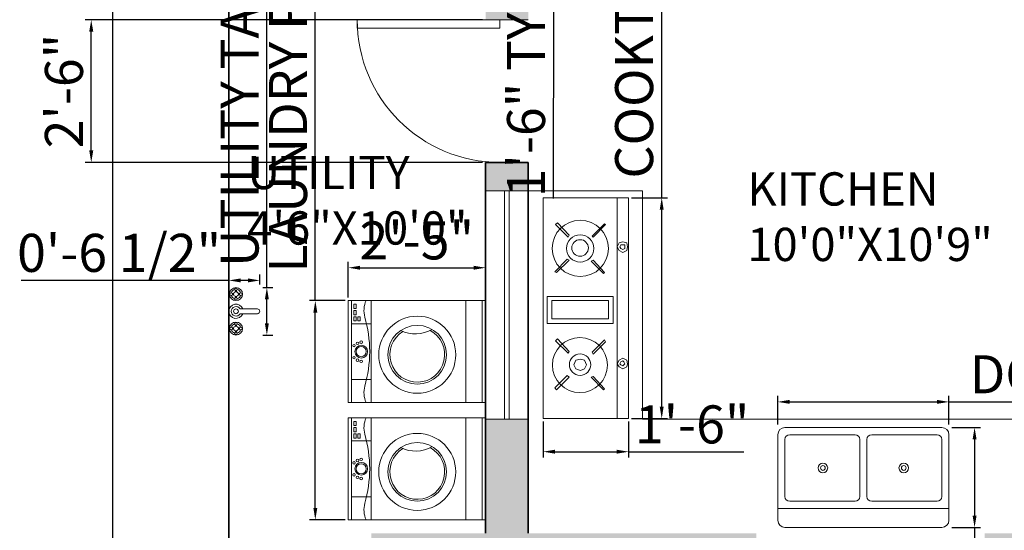
# Model space of a CAD drawing. Units: inches. Extents: x 4732 to 5926, y 2665 to 3255.
# Tile 2 of 8: x 4774 to 4982, y 2827 to 2934. Entities that reach past the tile are written whole.
import ezdxf

# ---------------------------------------------------------------- set-up
doc = ezdxf.new("R2010")
doc.units = ezdxf.units.IN
for name, color, linetype, lineweight in [('A-ANNO-DIMS', 2, 'Continuous', 18), ('A-AREA-IDEN', 7, 'Continuous', 18), ('A-DOOR', 3, 'Continuous', 18), ('A-EQPM', 8, 'Continuous', 18), ('A-FLOR-CASE', 7, 'Continuous', 18), ('A-GLAZ', 4, 'Continuous', 18), ('A-WALL', 7, 'Continuous', 35), ('A-WALL-PATT', 8, 'Continuous', 13), ('C-PROP', 7, 'Continuous', 35), ('Сантехника', 7, 'Continuous', 18)]:
    doc.layers.add(name, color=color, linetype=linetype, lineweight=lineweight)
doc.styles.get("Standard").update_dxf_attribs({"font": 'arial.ttf'})
doc.dimstyles.new('ISO-25', dxfattribs={"dimtxt": 8, "dimasz": 2.5, "dimexe": 1.25, "dimexo": 0.625, "dimtad": 1, "dimdec": 1, "dimlunit": 3, "dimtxsty": 'Standard', "dimcen": 2.5, "dimadec": 0, "dimazin": 0, "dimtfac": 1, "dimtdec": 1, "dimtmove": 0, "dimatfit": 3, "dimfxl": 1, "dimarcsym": 0})

# ---------------------------------------------------------------- blocks, each defined once
blk = doc.blocks.new('Sink-double - 36 in top')
for p, q in [((-18, -4), (18, -4)), ((-0.75, -18.5), (-0.75, -6.5)), ((0.75, -6.5), (0.75, -18.5))]:
    blk.add_line(p, q)
for points in [[(-16.5, 0), (16.5, 0)], [(-18, -19.5), (-18, -1.5)], [(18, -1.5), (18, -19.5)], [(-15.5, -5.5), (-1.75, -5.5)], [(1.75, -5.5), (15.5, -5.5)], [(-16.5, -18.5), (-16.5, -6.5)], [(16.5, -6.5), (16.5, -18.5)], [(-1.75, -19.5), (-15.5, -19.5)], [(15.5, -19.5), (1.75, -19.5)], [(16.5, -21), (-16.5, -21)]]:
    blk.add_lwpolyline(points)
for centre, radius in [((-8.5, -12.5), 1), ((-8.5, -12.5), 0.5), ((8.5, -12.5), 1), ((8.5, -12.5), 0.5)]:
    blk.add_circle(centre, radius)
for centre, radius, start, end in [((-16.5, -1.5), 1.5, 90, 180), ((16.5, -1.5), 1.5, 0, 90), ((-15.5, -6.5), 1, 90, 180), ((-1.75, -6.5), 1, 0, 90), ((1.75, -6.5), 1, 90, 180), ((15.5, -6.5), 1, 0, 90), ((-15.5, -18.5), 1, 180, 270), ((-1.75, -18.5), 1, 270, 0), ((1.75, -18.5), 1, 180, 270), ((15.5, -18.5), 1, 270, 0), ((-16.5, -19.5), 1.5, 180, 270), ((16.5, -19.5), 1.5, 270, 0)]:
    blk.add_arc(centre, radius, start, end)
blk = doc.blocks.new('wash')
at = {"layer": 'Сантехника'}
for p, q in [((4817.13, 2840.92), (4788.24, 2840.92)), ((4788.24, 2819.46), (4788.24, 2840.92)), ((4788.93, 2819.46), (4788.93, 2840.92)), ((4793.08, 2819.46), (4793.08, 2840.92)), ((4812.98, 2819.46), (4812.98, 2840.92)), ((4816.44, 2819.46), (4816.44, 2840.92)), ((4817.13, 2819.46), (4817.13, 2840.92)), ((4793.08, 2836.07), (4788.93, 2836.07)), ((4793.08, 2824.31), (4788.93, 2824.31)), ((4817.13, 2819.46), (4788.24, 2819.46)), ((4817.13, 2816.27), (4788.24, 2816.27)), ((4788.24, 2794.82), (4788.24, 2816.27)), ((4788.93, 2794.82), (4788.93, 2816.27)), ((4793.08, 2794.82), (4793.08, 2816.27)), ((4812.98, 2794.82), (4812.98, 2816.27)), ((4816.44, 2794.82), (4816.44, 2816.27)), ((4817.13, 2794.82), (4817.13, 2816.27)), ((4793.08, 2811.43), (4788.93, 2811.43)), ((4793.08, 2799.66), (4788.93, 2799.66)), ((4817.13, 2794.82), (4788.24, 2794.82))]:
    blk.add_line(p, q, dxfattribs=at)
for points in [[(4789.4, 2839.27), (4789.4, 2840.17), (4789.9, 2840.17), (4789.9, 2839.27)], [(4789.4, 2837.95), (4789.4, 2838.85), (4789.9, 2838.85), (4789.9, 2837.95)], [(4789.4, 2836.64), (4789.4, 2837.53), (4789.9, 2837.53), (4789.9, 2836.64)], [(4790.27, 2836.64), (4790.27, 2837.53), (4790.77, 2837.53), (4790.77, 2836.64)], [(4789.4, 2814.62), (4789.4, 2815.52), (4789.9, 2815.52), (4789.9, 2814.62)], [(4789.4, 2813.31), (4789.4, 2814.2), (4789.9, 2814.2), (4789.9, 2813.31)], [(4789.4, 2811.99), (4789.4, 2812.89), (4789.9, 2812.89), (4789.9, 2811.99)], [(4790.27, 2811.99), (4790.27, 2812.89), (4790.77, 2812.89), (4790.77, 2811.99)]]:
    blk.add_lwpolyline(points, close=True, dxfattribs=at)
for centre, radius in [((4802.77, 2829.54), 8.1), ((4802.77, 2829.54), 6.17), ((4790.19, 2831.93), 0.271), ((4790.98, 2832.18), 0.271), ((4789.46, 2831.45), 0.271), ((4790.98, 2830.19), 1.34), ((4790.98, 2830.19), 1.07), ((4789.46, 2828.92), 0.271), ((4790.19, 2828.4), 0.271), ((4790.98, 2828.15), 0.271), ((4802.77, 2804.9), 8.1), ((4802.77, 2804.9), 6.17), ((4789.46, 2806.8), 0.271), ((4790.19, 2807.28), 0.271), ((4790.98, 2807.53), 0.271), ((4790.98, 2805.55), 1.34), ((4790.98, 2805.55), 1.07), ((4789.46, 2804.27), 0.271), ((4790.19, 2803.75), 0.271), ((4790.98, 2803.5), 0.271)]:
    blk.add_circle(centre, radius, dxfattribs=at)
for centre, radius, start, end in [((4796.44, 2838.85), 4.89, 154.895, 196.6068), ((4762.87, 2829.66), 29.92, 1.0206, 15.0937), ((4802.77, 2829.54), 5.77, 121.8067, 62.1506), ((4802.39, 2840.74), 6.83, 243.19, 300.7673), ((4762.87, 2830.72), 29.92, 344.9063, 358.9794), ((4796.44, 2821.54), 4.89, 163.3932, 205.105), ((4796.44, 2814.2), 4.89, 154.895, 196.6068), ((4762.87, 2805.01), 29.92, 1.0206, 15.0937), ((4802.77, 2804.9), 5.77, 121.8067, 62.1506), ((4802.39, 2816.1), 6.83, 243.19, 300.7673), ((4762.87, 2806.08), 29.92, 344.9063, 358.9794), ((4796.44, 2796.89), 4.89, 163.3932, 205.105)]:
    blk.add_arc(centre, radius, start, end, dxfattribs=at)
blk = doc.blocks.new('gas 1')
for points in [[(35.93, -1.87), (35.93, 0), (0, 0), (0, -1.87)], [(8.12, -0.94), (8.44, -1.56), (8.91, -1.87), (9.53, -1.56), (9.84, -0.94), (9.53, -0.31), (8.91, -0.16), (8.44, -0.31)], [(8.59, -0.94), (8.75, -1.25), (8.91, -1.41), (9.22, -1.25), (9.37, -0.94), (9.22, -0.78), (8.91, -0.62), (8.75, -0.78)], [(27.03, -0.94), (27.34, -1.56), (27.97, -1.87), (28.59, -1.56), (28.75, -0.94), (28.59, -0.31), (27.97, -0.16), (27.34, -0.31)], [(27.5, -0.94), (27.65, -1.25), (27.97, -1.41), (28.28, -1.25), (28.28, -0.94), (28.28, -0.62), (27.97, -0.62), (27.65, -0.62)], [(19.84, -13.28), (15.47, -13.28), (15.47, -2.5), (19.84, -2.5)], [(4.84, -3.91), (4.69, -4.06), (6.72, -6.09), (6.87, -5.78)], [(12.81, -3.91), (12.5, -3.75), (10.47, -5.78), (10.78, -5.94)], [(19.22, -12.5), (16.25, -12.5), (16.25, -3.28), (19.22, -3.28)], [(23.75, -3.91), (23.59, -4.06), (25.62, -6.09), (25.78, -5.78)], [(31.71, -3.91), (31.56, -3.75), (29.53, -5.78), (29.68, -5.94)], [(7.81, -7.81), (8.12, -8.59), (8.75, -8.91), (9.53, -8.59), (9.69, -7.81), (9.53, -7.19), (8.75, -6.87), (8.12, -7.19)], [(7.03, -10), (6.72, -9.69), (4.69, -11.72), (5, -12.03)], [(12.97, -11.56), (10.94, -9.69), (10.62, -9.84), (12.65, -11.87)], [(23.75, -11.72), (23.9, -12.03), (25.93, -10), (25.78, -9.69)], [(31.87, -11.56), (29.84, -9.69), (29.53, -9.84), (31.56, -11.87)]]:
    blk.add_lwpolyline(points, close=True)
blk.add_lwpolyline([(35.93, -1.87), (35.93, -13.9), (0, -13.9), (0, -1.87)])
for centre, radius in [((8.7, -7.92), 4.48), ((27.7, -7.86), 4.58), ((8.77, -7.89), 1.74), ((27.69, -7.89), 2.22), ((27.76, -7.89), 1.35)]:
    blk.add_circle(centre, radius)
blk = doc.blocks.new('*U19')
for p, q in [((0, 0), (0, -6)), ((30, 0), (30, -6))]:
    blk.add_line(p, q)
blk.add_lwpolyline([(0, 0), (0, 30), (1.75, 30), (1.75, 0)], close=True)
blk.add_arc((0, 0), 30, 0, 90)
blk = doc.blocks.new('*D28')
at = {"layer": 'A-ANNO-DIMS', "color": 0, "lineweight": -2, "transparency": 16777216}
for p, q in [((4817.76, 3215.93), (4792.67, 3215.93)), ((4793.92, 3213.43), (4793.92, 2738.43)), ((4817.76, 2735.93), (4792.67, 2735.93))]:
    blk.add_line(p, q, dxfattribs=at)
at = {"layer": 'A-ANNO-DIMS', "color": 0, "transparency": 16777216}
for points in [[(4793.5, 3213.43), (4794.33, 3213.43), (4793.92, 3215.93)], [(4793.5, 2738.43), (4794.33, 2738.43), (4793.92, 2735.93)]]:
    blk.add_solid(points, dxfattribs=at)
at = {"layer": 'Defpoints', "color": 0, "transparency": 16777216}
for p in [(4818.38, 3215.93), (4793.92, 2735.93), (4818.38, 2735.93)]:
    blk.add_point(p, dxfattribs=at)
at = {"layer": 'A-ANNO-DIMS', "color": 0, "transparency": 16777216, "insert": (4789.21, 2975.93), "char_height": 8, "attachment_point": 5, "rotation": 90}
blk.add_mtext("40'", dxfattribs=at)
blk = doc.blocks.new('Faucet - Bathroom top')
for p, q in [((-4.107, 0.125), (-4.375, 0.125)), ((-3.75, 0.4788), (-3.75, 0.75)), ((-3.5, 0.482), (-3.5, 0.75)), ((-3.1461, 0.125), (-2.875, 0.125)), ((3.143, 0.125), (2.875, 0.125)), ((3.5, 0.4788), (3.5, 0.75)), ((3.75, 0.482), (3.75, 0.75)), ((4.1039, 0.125), (4.375, 0.125)), ((-4.1039, -0.125), (-4.375, -0.125)), ((-3.75, -0.4821), (-3.75, -0.75)), ((-3.5, -0.4789), (-3.5, -0.75)), ((-3.143, -0.125), (-2.875, -0.125)), ((-0.5, -0.8639), (-0.5, -4.5)), ((0.5, -4.5), (0.5, -0.8631)), ((3.1461, -0.125), (2.875, -0.125)), ((3.5, -0.4821), (3.5, -0.75)), ((3.75, -0.4789), (3.75, -0.75)), ((4.107, -0.125), (4.375, -0.125))]:
    blk.add_line(p, q)
for centre, radius in [((-3.625, 0), 1.375), ((-4.625, 0), 0.2795), ((-3.625, 0), 0.5), ((-3.625, 1), 0.2795), ((-2.625, 0), 0.2795), ((0, 0), 0.5), ((3.625, 0), 1.375), ((2.625, 0), 0.2795), ((3.625, 0), 0.5), ((3.625, 1), 0.2795), ((4.625, 0), 0.2795), ((-3.625, -1), 0.2795), ((3.625, -1), 0.2795)]:
    blk.add_circle(centre, radius)
for centre, radius, start, end in [((-3.625, 0), 1, 105.2407, 164.2093), ((-3.625, 0), 1, 16.44125, 74.07887), ((0, 0), 1.5, 289.6514, 250.3603), ((0, 0), 1, 300.3431, 239.7554), ((3.625, 0), 1, 106.12, 164.0884), ((3.625, 0), 1, 16.23422, 73.90469), ((-3.625, 0), 1, 196.2342, 253.9047), ((-3.625, 0), 1, 286.12, 344.0884), ((3.625, 0), 1, 196.4413, 254.0789), ((3.625, 0), 1, 285.2407, 344.2093), ((0, -4.5), 0.5, 180, 0)]:
    blk.add_arc(centre, radius, start, end)
blk = doc.blocks.new('GLAZ-UNIT-48IN')
for p, q in [((0, 1), (48, 1)), ((0, 0), (48, 0))]:
    blk.add_line(p, q)
blk = doc.blocks.new('COUNTER-KITCHEN-L')
for p, q in [((0, 48), (24, 48)), ((24, 0), (24, 48)), ((24, 0), (120, 0))]:
    blk.add_line(p, q)
blk = doc.blocks.new('*D77')
at = {"layer": 'A-ANNO-DIMS', "color": 0, "lineweight": -2, "transparency": 16777216}
for p, q in [((4888.93, 2966.23), (4885.41, 2966.23)), ((4886.66, 2963.73), (4886.66, 2950.62)), ((4888.92, 2948.12), (4885.4, 2948.12)), ((4886.65, 2948.12), (4886.64, 2896.36))]:
    blk.add_line(p, q, dxfattribs=at)
at = {"layer": 'A-ANNO-DIMS', "color": 0, "transparency": 16777216}
for points in [[(4886.24, 2963.73), (4887.08, 2963.73), (4886.66, 2966.23)], [(4886.24, 2950.62), (4887.07, 2950.62), (4886.65, 2948.12)]]:
    blk.add_solid(points, dxfattribs=at)
at = {"layer": 'Defpoints', "color": 0, "transparency": 16777216}
for p in [(4889.55, 2966.23), (4886.65, 2948.12), (4889.55, 2948.12)]:
    blk.add_point(p, dxfattribs=at)
at = {"layer": 'A-ANNO-DIMS', "color": 0, "transparency": 16777216, "insert": (4881.94, 2920.99), "char_height": 8, "attachment_point": 5, "rotation": 89.9851}
blk.add_mtext('1\'-6" TYP.', dxfattribs=at)
blk = doc.blocks.new('*D84')
at = {"layer": 'A-ANNO-DIMS', "color": 0, "lineweight": -2, "transparency": 16777216}
for p, q in [((4933.87, 2848.78), (4933.87, 2854.8)), ((4969.87, 2848.78), (4969.87, 2854.8)), ((4936.37, 2853.55), (4967.37, 2853.55)), ((4969.87, 2853.55), (5072.74, 2853.55))]:
    blk.add_line(p, q, dxfattribs=at)
at = {"layer": 'A-ANNO-DIMS', "color": 0, "transparency": 16777216}
for points in [[(4936.37, 2853.97), (4936.37, 2853.14), (4933.87, 2853.55)], [(4967.37, 2853.97), (4967.37, 2853.14), (4969.87, 2853.55)]]:
    blk.add_solid(points, dxfattribs=at)
at = {"layer": 'Defpoints', "color": 0, "transparency": 16777216}
for p in [(4969.87, 2853.55), (4933.87, 2848.15), (4969.87, 2848.15)]:
    blk.add_point(p, dxfattribs=at)
at = {"layer": 'A-ANNO-DIMS', "color": 0, "transparency": 16777216, "insert": (5022.55, 2858.32), "char_height": 8, "attachment_point": 5}
blk.add_mtext('DOUBLE SINK 3\'-0"', dxfattribs=at)
blk = doc.blocks.new('*D85')
at = {"layer": 'A-ANNO-DIMS', "color": 0, "lineweight": -2, "transparency": 16777216}
for p, q in [((4970.49, 2848.15), (4976.52, 2848.15)), ((4975.27, 2845.65), (4975.27, 2829.65)), ((4970.49, 2827.15), (4976.52, 2827.15)), ((4975.27, 2827.15), (4975.27, 2802.89))]:
    blk.add_line(p, q, dxfattribs=at)
at = {"layer": 'A-ANNO-DIMS', "color": 0, "transparency": 16777216}
for points in [[(4974.85, 2845.65), (4975.69, 2845.65), (4975.27, 2848.15)], [(4974.85, 2829.65), (4975.69, 2829.65), (4975.27, 2827.15)]]:
    blk.add_solid(points, dxfattribs=at)
at = {"layer": 'Defpoints', "color": 0, "transparency": 16777216}
for p in [(4969.87, 2848.15), (4969.87, 2827.15), (4975.27, 2827.15)]:
    blk.add_point(p, dxfattribs=at)
at = {"layer": 'A-ANNO-DIMS', "color": 0, "transparency": 16777216, "insert": (4970.56, 2813.77), "char_height": 8, "attachment_point": 5, "rotation": 90}
blk.add_mtext('1\'-9"', dxfattribs=at)
blk = doc.blocks.new('*D86')
at = {"layer": 'A-ANNO-DIMS', "color": 0, "lineweight": -2, "transparency": 16777216}
for p, q in [((4836.57, 2874.85), (4836.57, 2991.43)), ((4842.86, 2874.85), (4835.32, 2874.85)), ((4836.57, 2831.25), (4836.57, 2872.35)), ((4842.86, 2828.75), (4835.32, 2828.75))]:
    blk.add_line(p, q, dxfattribs=at)
at = {"layer": 'A-ANNO-DIMS', "color": 0, "transparency": 16777216}
for points in [[(4836.16, 2872.35), (4836.99, 2872.35), (4836.57, 2874.85)], [(4836.16, 2831.25), (4836.99, 2831.25), (4836.57, 2828.75)]]:
    blk.add_solid(points, dxfattribs=at)
at = {"layer": 'Defpoints', "color": 0, "transparency": 16777216}
for p in [(4836.57, 2874.85), (4843.49, 2874.85), (4843.49, 2828.75)]:
    blk.add_point(p, dxfattribs=at)
at = {"layer": 'A-ANNO-DIMS', "color": 0, "transparency": 16777216, "insert": (4831.86, 2934.39), "char_height": 8, "attachment_point": 5, "rotation": 90}
blk.add_mtext('LAUNDRY PAIR 3\'-10"', dxfattribs=at)
blk = doc.blocks.new('*D87')
at = {"layer": 'A-ANNO-DIMS', "color": 0, "lineweight": -2, "transparency": 16777216}
for p, q in [((4843.49, 2875.48), (4843.49, 2883.02)), ((4845.99, 2881.77), (4869.88, 2881.77)), ((4872.38, 2875.48), (4872.38, 2883.02))]:
    blk.add_line(p, q, dxfattribs=at)
at = {"layer": 'A-ANNO-DIMS', "color": 0, "transparency": 16777216}
for points in [[(4845.99, 2882.18), (4845.99, 2881.35), (4843.49, 2881.77)], [(4869.88, 2882.18), (4869.88, 2881.35), (4872.38, 2881.77)]]:
    blk.add_solid(points, dxfattribs=at)
at = {"layer": 'Defpoints', "color": 0, "transparency": 16777216}
for p in [(4872.38, 2881.77), (4843.49, 2874.85), (4872.38, 2874.85)]:
    blk.add_point(p, dxfattribs=at)
at = {"layer": 'A-ANNO-DIMS', "color": 0, "transparency": 16777216, "insert": (4857.93, 2886.48), "char_height": 8, "attachment_point": 5}
blk.add_mtext('2\'-5"', dxfattribs=at)
blk = doc.blocks.new('*D90')
at = {"layer": 'A-ANNO-DIMS', "color": 0, "lineweight": -2, "transparency": 16777216}
for p, q in [((4909.45, 2896.49), (4909.45, 3005.26)), ((4903.1, 2896.49), (4910.7, 2896.49)), ((4909.45, 2852.54), (4909.45, 2893.99)), ((4903.1, 2850.04), (4910.7, 2850.04))]:
    blk.add_line(p, q, dxfattribs=at)
at = {"layer": 'A-ANNO-DIMS', "color": 0, "transparency": 16777216}
for points in [[(4909.03, 2893.99), (4909.86, 2893.99), (4909.45, 2896.49)], [(4909.03, 2852.54), (4909.86, 2852.54), (4909.45, 2850.04)]]:
    blk.add_solid(points, dxfattribs=at)
at = {"layer": 'Defpoints', "color": 0, "transparency": 16777216}
for p in [(4902.48, 2896.49), (4909.45, 2896.49), (4902.48, 2850.04)]:
    blk.add_point(p, dxfattribs=at)
at = {"layer": 'A-ANNO-DIMS', "color": 0, "transparency": 16777216, "insert": (4904.68, 2952.12), "char_height": 8, "attachment_point": 5, "rotation": 90}
blk.add_mtext('COOKTOP 3\'-10 1/2"', dxfattribs=at)
blk = doc.blocks.new('*D91')
at = {"layer": 'A-ANNO-DIMS', "color": 0, "lineweight": -2, "transparency": 16777216}
for p, q in [((4884.51, 2849.42), (4884.51, 2841.82)), ((4902.48, 2849.42), (4902.48, 2841.82)), ((4887.01, 2843.07), (4899.98, 2843.07)), ((4902.48, 2843.07), (4926.74, 2843.07))]:
    blk.add_line(p, q, dxfattribs=at)
at = {"layer": 'A-ANNO-DIMS', "color": 0, "transparency": 16777216}
for points in [[(4887.01, 2843.49), (4887.01, 2842.66), (4884.51, 2843.07)], [(4899.98, 2843.49), (4899.98, 2842.66), (4902.48, 2843.07)]]:
    blk.add_solid(points, dxfattribs=at)
at = {"layer": 'Defpoints', "color": 0, "transparency": 16777216}
for p in [(4884.51, 2850.04), (4902.48, 2850.04), (4902.48, 2843.07)]:
    blk.add_point(p, dxfattribs=at)
at = {"layer": 'A-ANNO-DIMS', "color": 0, "transparency": 16777216, "insert": (4915.86, 2847.78), "char_height": 8, "attachment_point": 5}
blk.add_mtext('1\'-6"', dxfattribs=at)
blk = doc.blocks.new('*D102')
at = {"layer": 'A-ANNO-DIMS', "color": 0, "lineweight": -2, "transparency": 16777216}
for p, q in [((4826.38, 2877.6), (4826.38, 2977.97)), ((4825.51, 2877.6), (4827.63, 2877.6)), ((4826.38, 2870.1), (4826.38, 2875.1)), ((4825.51, 2867.6), (4827.63, 2867.6))]:
    blk.add_line(p, q, dxfattribs=at)
at = {"layer": 'A-ANNO-DIMS', "color": 0, "transparency": 16777216}
for points in [[(4825.96, 2875.1), (4826.8, 2875.1), (4826.38, 2877.6)], [(4825.96, 2870.1), (4826.8, 2870.1), (4826.38, 2867.6)]]:
    blk.add_solid(points, dxfattribs=at)
at = {"layer": 'Defpoints', "color": 0, "transparency": 16777216}
for p in [(4824.88, 2877.6), (4826.38, 2877.6), (4824.88, 2867.6)]:
    blk.add_point(p, dxfattribs=at)
at = {"layer": 'A-ANNO-DIMS', "color": 0, "transparency": 16777216, "insert": (4821.67, 2929.03), "char_height": 8, "attachment_point": 5, "rotation": 90}
blk.add_mtext('UTILITY TAP 0\'-10"', dxfattribs=at)
blk = doc.blocks.new('*D103')
at = {"layer": 'A-ANNO-DIMS', "color": 0, "lineweight": -2, "transparency": 16777216}
for p, q in [((4818.38, 2878.23), (4818.38, 2880.35)), ((4824.88, 2878.23), (4824.88, 2880.35)), ((4818.38, 2879.1), (4774.72, 2879.1)), ((4822.38, 2879.1), (4820.88, 2879.1))]:
    blk.add_line(p, q, dxfattribs=at)
at = {"layer": 'A-ANNO-DIMS', "color": 0, "transparency": 16777216}
for points in [[(4820.88, 2879.52), (4820.88, 2878.68), (4818.38, 2879.1)], [(4822.38, 2879.52), (4822.38, 2878.68), (4824.88, 2879.1)]]:
    blk.add_solid(points, dxfattribs=at)
at = {"layer": 'Defpoints', "color": 0, "transparency": 16777216}
for p in [(4818.38, 2879.1), (4818.38, 2877.6), (4824.88, 2877.6)]:
    blk.add_point(p, dxfattribs=at)
at = {"layer": 'A-ANNO-DIMS', "color": 0, "transparency": 16777216, "insert": (4795.3, 2883.86), "char_height": 8, "attachment_point": 5}
blk.add_mtext('0\'-6 1/2"', dxfattribs=at)
blk = doc.blocks.new('*D106')
at = {"layer": 'A-ANNO-DIMS', "color": 0, "lineweight": -2, "transparency": 16777216}
for p, q in [((4871.76, 2933.93), (4788.18, 2933.93)), ((4789.43, 2906.43), (4789.43, 2931.43)), ((4871.76, 2903.93), (4788.18, 2903.93))]:
    blk.add_line(p, q, dxfattribs=at)
at = {"layer": 'A-ANNO-DIMS', "color": 0, "transparency": 16777216}
for points in [[(4789.01, 2931.43), (4789.85, 2931.43), (4789.43, 2933.93)], [(4789.01, 2906.43), (4789.85, 2906.43), (4789.43, 2903.93)]]:
    blk.add_solid(points, dxfattribs=at)
at = {"layer": 'Defpoints', "color": 0, "transparency": 16777216}
for p in [(4789.43, 2933.93), (4872.38, 2933.93), (4872.38, 2903.93)]:
    blk.add_point(p, dxfattribs=at)
at = {"layer": 'A-ANNO-DIMS', "color": 0, "transparency": 16777216, "insert": (4784.72, 2918.93), "char_height": 8, "attachment_point": 5, "rotation": 90}
blk.add_mtext('2\'-6"', dxfattribs=at)

msp = doc.modelspace()

# ---------------------------------------------------------------- hatches: boundary and pattern name
at = {"layer": 'A-WALL-PATT'}
h = msp.add_hatch(color=256, dxfattribs=at)
h.dxf.hatch_style = 1
h.paths.add_polyline_path([(4905.38, 3185.93), (4848.38, 3185.93), (4848.38, 3146.93), (4857.38, 3146.93), (4857.38, 3176.93), (4905.38, 3176.93)])
h.paths.add_polyline_path([(5022.38, 3185.93), (4953.38, 3185.93), (4953.38, 3176.93), (4966.1, 3176.93), (5001.38, 3176.93), (5001.38, 3098.93), (5028.38, 3098.93), (5028.38, 3104.93), (5007.38, 3104.93), (5007.38, 3176.93), (5022.38, 3176.93)])
h.paths.add_polyline_path([(5115.38, 3185.93), (5046.38, 3185.93), (5046.38, 3176.93), (5061.38, 3176.93), (5061.38, 3104.93), (5058.38, 3104.93), (5058.38, 3098.93), (5067.38, 3098.93), (5067.38, 3176.93), (5115.38, 3176.93)])
h.paths.add_polyline_path([(5220.38, 3185.93), (5163.38, 3185.93), (5163.38, 3176.93), (5168.97, 3176.93), (5211.38, 3176.93), (5211.38, 3146.93), (5220.38, 3146.93)])
h.paths.add_polyline_path([(4857.38, 3086.93), (4848.38, 3086.93), (4848.38, 3026.93), (4857.38, 3026.93), (4857.38, 3050.93), (5001.38, 3050.93), (5001.38, 3008.93), (5007.38, 3008.93), (5007.38, 3050.93), (5022.38, 3050.93), (5022.38, 3056.93), (4857.38, 3056.93)])
h.paths.add_polyline_path([(4857.38, 2978.93), (4848.38, 2978.93), (4848.38, 2945.93), (4872.38, 2945.93), (4872.38, 2933.93), (4875.38, 2933.93), (4881.38, 2933.93), (4881.38, 2954.93), (4857.38, 2954.93)])
h.paths.add_polyline_path([(4881.38, 2903.93), (4875.38, 2903.93), (4872.38, 2903.93), (4872.38, 2897.93), (4881.38, 2897.93)])
h.paths.add_polyline_path([(4881.38, 2849.93), (4872.38, 2849.93), (4872.38, 2828.75), (4872.38, 2825.93), (4848.38, 2825.93), (4848.38, 2804.93), (4857.38, 2804.93), (4857.38, 2816.93), (4929.38, 2816.93), (4929.38, 2825.93), (4881.38, 2825.93)])
h.paths.add_polyline_path([(4975.38, 2744.93), (4857.38, 2744.93), (4857.38, 2756.93), (4848.38, 2756.93), (4848.38, 2735.93), (4975.38, 2735.93)])
h.paths.add_polyline_path([(5160.38, 2915.93), (5160.38, 2918.93), (5007.38, 2918.93), (5007.38, 2960.93), (5001.38, 2960.93), (5001.38, 2825.93), (4977.38, 2825.93), (4977.38, 2816.93), (5010.38, 2816.93), (5010.38, 2909.93), (5160.38, 2909.93)])
h.paths.add_polyline_path([(5220.38, 2948.93), (5211.38, 2948.93), (5211.38, 2918.93), (5208.38, 2918.93), (5208.38, 2909.93), (5220.38, 2909.93)])
h.paths.add_polyline_path([(5220.38, 3086.93), (5211.38, 3086.93), (5211.38, 3056.93), (5106.38, 3056.93), (5106.38, 3050.93), (5211.38, 3050.93), (5211.38, 3020.93), (5220.38, 3020.93)])
h.paths.add_polyline_path([(5067.38, 3098.93), (5061.38, 3098.93), (5061.38, 3056.93), (5058.38, 3056.93), (5058.38, 3050.93), (5061.38, 3050.93), (5070.38, 3050.93), (5070.38, 3056.93), (5067.38, 3056.93)])
h.paths.add_polyline_path([(4883.76, 2941.13), (4938.24, 2941.13), (4938.24, 2949.38), (4883.76, 2949.38)], flags=9)
h.paths.add_polyline_path([(4840.48, 3026.79), (4840.48, 3093.88), (4825.54, 3093.88), (4825.54, 3026.79)], flags=9)
h.paths.add_polyline_path([(5245.66, 2994.98), (5245.66, 3062.07), (5230.72, 3062.07), (5230.72, 2994.98)], flags=9)
h.paths.add_polyline_path([(4994.89, 3193.24), (5061.99, 3193.24), (5061.99, 3208.18), (4994.89, 3208.18)], flags=9)
h.paths.add_polyline_path([(5081.53, 3115.35), (5081.53, 3161.13), (5073.28, 3161.13), (5073.28, 3115.35)], flags=25)
h.paths.add_polyline_path([(4997.53, 3115.35), (4997.53, 3161.13), (4989.28, 3161.13), (4989.28, 3115.35)], flags=25)
h.paths.add_polyline_path([(5175.31, 2866.04), (5202.42, 2866.04), (5202.42, 2876.71), (5175.31, 2876.71)], flags=9)
h.paths.add_polyline_path([(4820.13, 2876.28), (4869.1, 2876.28), (4869.1, 2902.89), (4820.13, 2902.89)], flags=9)
h.paths.add_polyline_path([(5104.69, 2868.81), (5158.82, 2868.81), (5158.82, 2895.42), (5104.69, 2895.42)], flags=25)
h.paths.add_polyline_path([(5084.11, 2966.75), (5138.25, 2966.75), (5138.25, 2993.36), (5084.11, 2993.36)], flags=9)
h.paths.add_polyline_path([(4897.84, 3000.24), (4946.81, 3000.24), (4946.81, 3026.85), (4897.84, 3026.85)], flags=9)
h.paths.add_polyline_path([(5009.53, 3133.48), (5059.32, 3133.48), (5059.32, 3160.09), (5009.53, 3160.09)], flags=9)
h.paths.add_polyline_path([(5124.24, 3088.37), (5180.47, 3088.37), (5180.47, 3114.99), (5124.24, 3114.99)], flags=9)
h.paths.add_polyline_path([(4897.52, 3088.37), (4965.52, 3088.37), (4965.52, 3114.99), (4897.52, 3114.99)], flags=9)
h.paths.add_polyline_path([(4924.5, 2879.19), (4978.63, 2879.19), (4978.63, 2905.8), (4924.5, 2905.8)], flags=9)

# ---------------------------------------------------------------- linework, layer by layer
at = {"layer": 'A-GLAZ'}
for p, q in [((4872.38, 2897.93), (4881.38, 2897.93)), ((4872.38, 2849.93), (4881.38, 2849.93))]:
    msp.add_line(p, q, dxfattribs=at)
at = {"layer": 'A-WALL'}
for p, q in [((4872.38, 2825.93), (4872.38, 2903.93)), ((4872.38, 2903.93), (4881.38, 2903.93)), ((4881.38, 2825.93), (4881.38, 2903.93))]:
    msp.add_line(p, q, dxfattribs=at)
at = {"layer": 'C-PROP'}
msp.add_lwpolyline([(4818.38, 3215.93), (5250.38, 3215.93), (5250.38, 2735.93), (4818.38, 2735.93)], close=True, dxfattribs=at)

# ---------------------------------------------------------------- block references
at = {"layer": 'A-DOOR', "xscale": -1, "rotation": 90}
msp.add_blockref('*U19', (4875.38, 2933.93), dxfattribs=at)
at = {"layer": 'A-EQPM', "xscale": -1.292580420916565, "yscale": 1.292580420916565, "zscale": 1.292580420916565, "rotation": 270}
msp.add_blockref('gas 1', (4902.48, 2850.04), dxfattribs=at)
at = {"layer": 'A-EQPM'}
msp.add_blockref('wash', (55.25, 33.93), dxfattribs=at)
at = {"layer": 'A-FLOR-CASE'}
msp.add_blockref('COUNTER-KITCHEN-L', (4881.38, 2849.93), dxfattribs=at)
at = {"layer": 'A-GLAZ', "rotation": 270}
msp.add_blockref('GLAZ-UNIT-48IN', (4876.38, 2897.93), dxfattribs=at)
at = {"layer": 'Сантехника', "rotation": 90}
msp.add_blockref('Faucet - Bathroom top', (4819.88, 2872.6), dxfattribs=at)
at = {"layer": 'Сантехника', "xscale": -1, "rotation": 180}
msp.add_blockref('Sink-double - 36 in top', (4951.87, 2827.15), dxfattribs=at)

# ---------------------------------------------------------------- texts
at = {"layer": 'A-AREA-IDEN', "char_height": 7, "attachment_point": 1}
for s, insert in [('{\\fTimes New Roman|b0|i0|c0|p18;UTILITY\\P4\'6"X10\'0"}', (4822.25, 2905.3)), ('{\\fTimes New Roman|b0|i0|c0|p18;KITCHEN\\P10\'0"X10\'9"}', (4927.46, 2901.84))]:
    msp.add_mtext_dynamic_manual_height_columns(s, width=61.0557, gutter_width=12.5, heights=[0], dxfattribs=dict(at, insert=insert))

# ---------------------------------------------------------------- dimensions: what is measured, and where the dimension line sits
at = {"layer": 'A-ANNO-DIMS'}
for base, p1, p2, angle, override, picture, middle in [((4793.92, 2735.93), (4818.38, 3215.93), (4818.38, 2735.93), 90, {"dimclrd": 0, "dimclre": 0, "dimclrt": 0}, '*D28', (4789.21, 2975.93)), ((4789.43, 2933.93), (4872.38, 2903.93), (4872.38, 2933.93), 90, {"dimdec": 1, "dimlfac": 1, "dimrnd": 0, "dimzin": 1, "dimdsep": 46, "dimlunit": 4, "dimfrac": 2}, '*D106', (4784.72, 2918.93)), ((4818.38, 2879.1), (4824.88, 2877.6), (4818.38, 2877.6), 180, {"dimdec": 1, "dimlfac": 1, "dimrnd": 0, "dimzin": 1, "dimdsep": 46, "dimlunit": 4, "dimfrac": 2}, '*D103', (4795.3, 2883.86)), ((4975.27, 2827.15), (4969.87, 2848.15), (4969.87, 2827.15), 270, {"dimdec": 1, "dimlfac": 1, "dimrnd": 0, "dimzin": 1, "dimdsep": 46, "dimlunit": 4, "dimfrac": 2}, '*D85', (4970.56, 2813.77))]:
    dim = msp.add_linear_dim(base=base, p1=p1, p2=p2, angle=angle, dimstyle='ISO-25', override=override, dxfattribs=at)
    dim.commit()
    dim.dimension.update_dxf_attribs({"geometry": picture, "text_midpoint": middle})
for base, p1, p2, angle, text, picture, middle in [((4909.4455, 2896.487), (4902.4785, 2850.0405), (4902.4785, 2896.487), 90, 'COOKTOP <>', '*D90', (4904.6786, 2952.1222)), ((4836.57, 2874.85), (4843.49, 2828.75), (4843.49, 2874.85), 90, 'LAUNDRY PAIR <>', '*D86', (4831.86, 2934.39)), ((4826.38, 2877.6), (4824.88, 2867.6), (4824.88, 2877.6), 90, 'UTILITY TAP <>', '*D102', (4821.67, 2929.03)), ((4886.65, 2948.12), (4889.55, 2966.23), (4889.55, 2948.12), 269.9851, '<> TYP.', '*D77', (4881.94, 2920.99))]:
    dim = msp.add_linear_dim(base=base, p1=p1, p2=p2, angle=angle, text=text, dimstyle='ISO-25', override={"dimdec": 1, "dimlfac": 1, "dimrnd": 0, "dimzin": 1, "dimdsep": 46, "dimlunit": 4, "dimfrac": 2}, dxfattribs=at)
    dim.commit()
    dim.dimension.update_dxf_attribs({"geometry": picture, "text_midpoint": middle})
for base, p1, p2, picture, middle in [((4872.38, 2881.77), (4843.49, 2874.85), (4872.38, 2874.85), '*D87', (4857.93, 2886.48)), ((4902.48, 2843.07), (4884.51, 2850.04), (4902.48, 2850.04), '*D91', (4915.86, 2847.78))]:
    dim = msp.add_linear_dim(base=base, p1=p1, p2=p2, dimstyle='ISO-25', override={"dimdec": 1, "dimlfac": 1, "dimrnd": 0, "dimzin": 1, "dimdsep": 46, "dimlunit": 4, "dimfrac": 2}, dxfattribs=at)
    dim.commit()
    dim.dimension.update_dxf_attribs({"geometry": picture, "text_midpoint": middle})
dim = msp.add_linear_dim(base=(4969.87, 2853.55), p1=(4933.87, 2848.15), p2=(4969.87, 2848.15), text='DOUBLE SINK <>', dimstyle='ISO-25', override={"dimdec": 1, "dimlfac": 1, "dimrnd": 0, "dimzin": 1, "dimdsep": 46, "dimlunit": 4, "dimfrac": 2}, dxfattribs=at)
dim.commit()
dim.dimension.update_dxf_attribs({"geometry": '*D84', "text_midpoint": (5022.55, 2858.32)})

doc.saveas('drawing.dxf')
